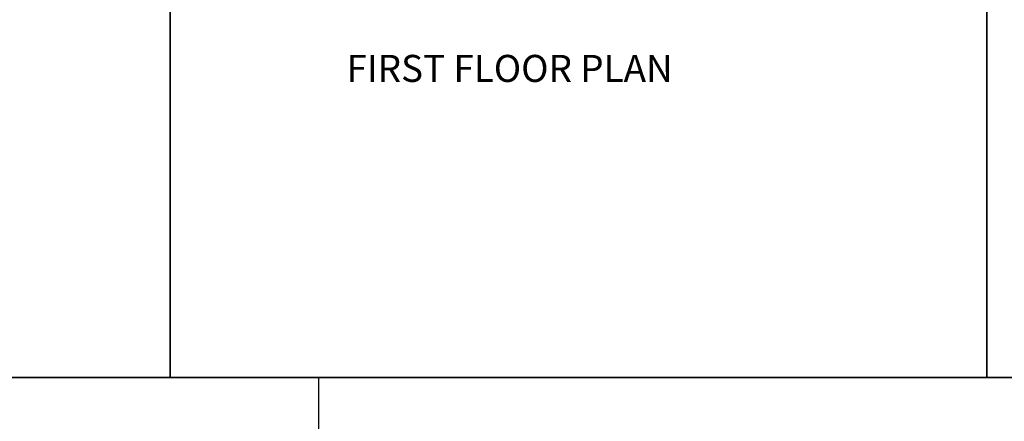
# Model space of a CAD drawing. Units: millimetres. Extents: x 20768 to 23556, y 50760 to 52704.
# Tile 14 of 36: x 21205 to 21642, y 51604 to 51783. Entities that reach past the tile are written whole.
import ezdxf

# ---------------------------------------------------------------- set-up
doc = ezdxf.new("R2010")
doc.units = ezdxf.units.MM
for name, color, linetype, lineweight in [('A-ANNO-TEXT', 7, 'Continuous', 18), ('A-ANNO-TTLB', 7, 'Continuous', 35), ('A-ELEV', 7, 'Continuous', 25)]:
    doc.layers.add(name, color=color, linetype=linetype, lineweight=lineweight)
doc.styles.get("Standard").update_dxf_attribs({"font": 'arial.ttf'})

msp = doc.modelspace()

# ---------------------------------------------------------------- linework, layer by layer
at = {"layer": 'A-ANNO-TTLB'}
for p, q in [((21271.86, 52703.98), (21271.86, 51623.53)), ((21634.36, 52703.98), (21634.36, 51623.53))]:
    msp.add_line(p, q, dxfattribs=at)
msp.add_lwpolyline([(20768.14, 52703.98), (23555.8, 52703.98), (23555.8, 51623.53), (20768.14, 51623.53)], close=True, dxfattribs=at)
at = {"layer": 'A-ELEV'}
msp.add_line((21337.76, 51623.53), (21337.76, 50975.78), dxfattribs=at)

# ---------------------------------------------------------------- texts
at = {"layer": 'A-ANNO-TEXT', "insert": (21350.17, 51766.88), "char_height": 12, "attachment_point": 1}
msp.add_mtext_dynamic_manual_height_columns('FIRST FLOOR PLAN', width=206.7681, gutter_width=12.5, heights=[0], dxfattribs=at)

doc.saveas('drawing.dxf')
